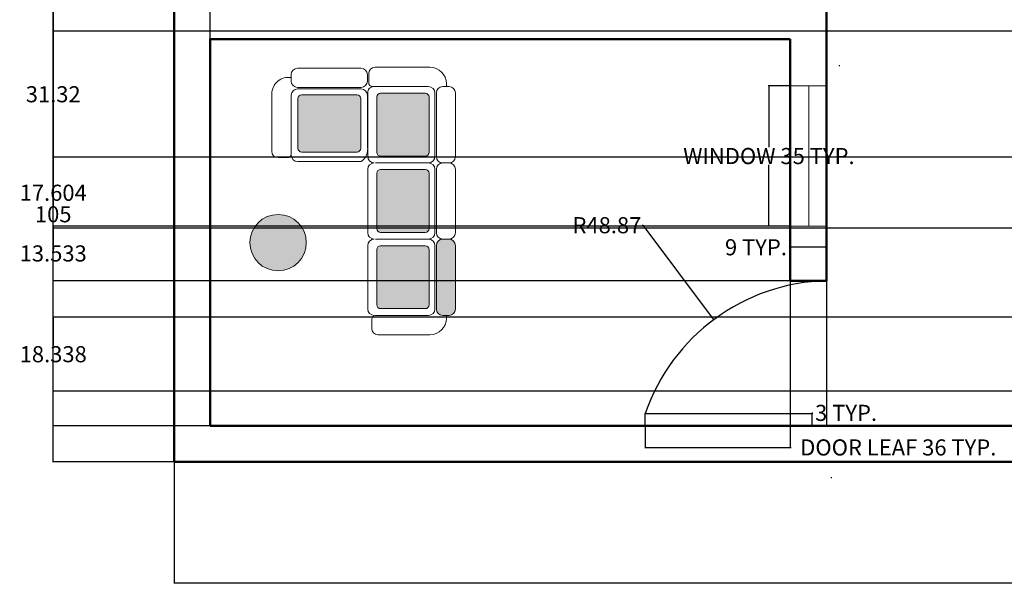
# Model space of a CAD drawing. Units: inches. Extents: x 1454 to 2136, y 626 to 1213.
# Tile 1 of 23: x 1454 to 1699, y 626 to 768. Entities that reach past the tile are written whole.
import ezdxf

# ---------------------------------------------------------------- set-up
doc = ezdxf.new("R2010")
doc.units = ezdxf.units.IN
doc.header["$MEASUREMENT"] = 0
for name, color, linetype, lineweight in [('A-ANNO-DIMS', 2, 'Continuous', 18), ('A-DOOR', 3, 'Continuous', 25), ('A-FURN', 9, 'Continuous', 18), ('A-FURN-PATT', 252, 'Continuous', 13), ('A-GLAZ', 4, 'Continuous', 18), ('A-PLNT-PATT', 116, 'Continuous', 13), ('A-WALL', 7, 'Continuous', 50), ('sofa', 4, 'Continuous', 18)]:
    doc.layers.add(name, color=color, linetype=linetype, lineweight=lineweight)
doc.styles.get("Standard").update_dxf_attribs({"font": 'arial.ttf'})
doc.dimstyles.get("Standard").update_dxf_attribs({"dimtxt": 4, "dimasz": 0.18, "dimexe": 0.18, "dimexo": 0.0625, "dimgap": 0.09, "dimtad": 0, "dimtih": 1, "dimtoh": 1, "dimdec": 0, "dimrnd": 6, "dimzin": 0, "dimdsep": 46, "dimlunit": 3, "dimtxsty": 'Standard', "dimcen": 0.09, "dimadec": 0, "dimazin": 0, "dimtfac": 1, "dimtdec": 0, "dimtofl": 0, "dimtmove": 0, "dimatfit": 3, "dimfxl": 1, "dimtolj": 1, "dimtzin": 0, "dimarcsym": 0})

# ---------------------------------------------------------------- blocks, each defined once
blk = doc.blocks.new('A$C611E44E9')
for p, q in [((0.6611, 1.4447), (0.2101, 1.4447)), ((0.7111, 1.3223), (0.7111, 1.3947)), ((0.0084, 1.2424), (0.0084, 0.7424)), ((0.1084, 1.2927), (0.0584, 1.2927)), ((0.0584, 1.2924), (0.1084, 1.2924)), ((0.1584, 1.2424), (0.1584, 0.7424)), ((0.1705, 1.2422), (0.1705, 0.7424)), ((0.6811, 1.2924), (0.2205, 1.2924)), ((0.6811, 1.2924), (0.2205, 1.2924)), ((0.6811, 1.2922), (0.2205, 1.2922)), ((0.2465, 1.2392), (0.6374, 1.2392)), ((0.7418, 0.7424), (0.7418, 1.2422)), ((0.2165, 0.7749), (0.2165, 1.2092)), ((0.6674, 1.2092), (0.6674, 0.7749)), ((0.6374, 0.7449), (0.2465, 0.7449)), ((0, 0.6327), (0, 0.2017)), ((0.1224, 0.6827), (0.05, 0.6827)), ((0.1084, 0.6927), (0.0584, 0.6927)), ((0.0584, 0.6924), (0.1084, 0.6924)), ((0.1524, 0.6527), (0.1524, 0.2121)), ((0.2024, 0.6896), (0.7021, 0.6896)), ((0.6373, 0.6924), (0.2205, 0.6924)), ((0.6373, 0.6924), (0.2205, 0.6924)), ((0.7521, 0.6289), (0.7521, 0.2121)), ((0.7521, 0.6289), (0.7521, 0.2121)), ((0.8021, 0.6896), (1.3018, 0.6896)), ((1.3521, 0.6289), (1.3521, 0.2121)), ((1.3521, 0.6289), (1.3521, 0.2121)), ((1.4021, 0.6896), (1.9018, 0.6896)), ((1.9518, 0.6289), (1.9518, 0.2121)), ((1.952, 0.6289), (1.952, 0.2121)), ((1.982, 0.6589), (2.0543, 0.6589)), ((0.2048, 0.5892), (0.2048, 0.2381)), ((0.6691, 0.6192), (0.2348, 0.6192)), ((0.6991, 0.2381), (0.6991, 0.5892)), ((0.8045, 0.5892), (0.8045, 0.2381)), ((1.2688, 0.6192), (0.8345, 0.6192)), ((1.2988, 0.2381), (1.2988, 0.5892)), ((1.4045, 0.5892), (1.4045, 0.2381)), ((1.8688, 0.6192), (1.4345, 0.6192)), ((1.8988, 0.2381), (1.8988, 0.5892)), ((2.1043, 0.6089), (2.1043, 0.2017)), ((0.7021, 0.1621), (0.2024, 0.1621)), ((0.2348, 0.2081), (0.6691, 0.2081)), ((1.3018, 0.1621), (0.8021, 0.1621)), ((0.8345, 0.2081), (1.2688, 0.2081)), ((1.9018, 0.1621), (1.4021, 0.1621)), ((1.4345, 0.2081), (1.8688, 0.2081)), ((0.1524, 0.05), (0.1524, 0.1)), ((0.7024, 0.15), (0.2024, 0.15)), ((0.7521, 0.05), (0.7521, 0.1)), ((0.7524, 0.1), (0.7524, 0.05)), ((1.3021, 0.15), (0.8021, 0.15)), ((1.3521, 0.05), (1.3521, 0.1)), ((1.3524, 0.1), (1.3524, 0.05)), ((1.9021, 0.15), (1.4021, 0.15)), ((1.952, 0.05), (1.952, 0.1)), ((1.9521, 0.1), (1.9521, 0.05)), ((0.13, 0.0717), (0.15, 0.0717)), ((0.7024, 0), (0.2024, 0)), ((1.3021, 0), (0.8021, 0)), ((1.9021, 0), (1.4021, 0)), ((1.9743, 0.0717), (1.9543, 0.0717))]:
    blk.add_line(p, q)
for centre, radius, start, end in [((0.2101, 1.3147), 0.13, 90, 189.86144), ((0.6611, 1.3947), 0.05, 0, 90), ((0.6811, 1.3223), 0.03, 270, 0), ((0.0584, 1.2424), 0.05, 90, 180), ((0.1084, 1.2424), 0.05, 0, 90), ((0.2205, 1.2422), 0.05, 90, 180), ((0.2465, 1.2092), 0.03, 90, 180), ((0.6374, 1.2092), 0.03, 0, 90), ((0.6918, 1.2422), 0.05, 0, 90), ((0.2465, 0.7749), 0.03, 180, 270), ((0.6374, 0.7749), 0.03, 270, 0), ((0.0584, 0.7424), 0.05, 180, 270), ((0.1084, 0.7424), 0.05, 270, 0), ((0.2205, 0.7424), 0.05, 180, 270), ((0.653, 0.796), 0.1037, 267.24891, 328.87945), ((0.05, 0.6327), 0.05, 90, 180), ((0.1224, 0.6527), 0.03, 0, 90), ((0.1981, 0.6441), 0.0458, 84.66489, 178.99029), ((0.7021, 0.6396), 0.05, 0, 90), ((0.8021, 0.6396), 0.05, 90, 180), ((1.3018, 0.6396), 0.05, 0, 90), ((1.4021, 0.6396), 0.05, 90, 180), ((1.9018, 0.6396), 0.05, 0, 90), ((1.982, 0.6289), 0.03, 90, 180), ((2.0543, 0.6089), 0.05, 0, 90), ((0.2348, 0.5892), 0.03, 90, 180), ((0.6691, 0.5892), 0.03, 0, 90), ((0.8345, 0.5892), 0.03, 90, 180), ((1.2688, 0.5892), 0.03, 0, 90), ((1.4345, 0.5892), 0.03, 90, 180), ((1.8688, 0.5892), 0.03, 0, 90), ((0.2348, 0.2381), 0.03, 180, 270), ((0.6691, 0.2381), 0.03, 270, 0), ((0.8345, 0.2381), 0.03, 180, 270), ((1.2688, 0.2381), 0.03, 270, 0), ((1.4345, 0.2381), 0.03, 180, 270), ((1.8688, 0.2381), 0.03, 270, 0), ((0.13, 0.2017), 0.13, 180, 270), ((0.2024, 0.2121), 0.05, 180, 270), ((0.7021, 0.2121), 0.05, 270, 0), ((0.8021, 0.2121), 0.05, 180, 270), ((1.3018, 0.2121), 0.05, 270, 0), ((1.4021, 0.2121), 0.05, 180, 270), ((1.9018, 0.2121), 0.05, 270, 0), ((1.9743, 0.2017), 0.13, 270, 0), ((0.2024, 0.1), 0.05, 90, 180), ((0.7024, 0.1), 0.05, 0, 90), ((0.8021, 0.1), 0.05, 90, 180), ((1.3021, 0.1), 0.05, 0, 90), ((1.4021, 0.1), 0.05, 90, 180), ((1.9021, 0.1), 0.05, 0, 90), ((0.2024, 0.05), 0.05, 180, 270), ((0.7024, 0.05), 0.05, 270, 0), ((0.8021, 0.05), 0.05, 180, 270), ((1.3021, 0.05), 0.05, 270, 0), ((1.4021, 0.05), 0.05, 180, 270), ((1.9021, 0.05), 0.05, 270, 0)]:
    blk.add_arc(centre, radius, start, end)
blk = doc.blocks.new('WIN-34_84')
blk.add_line((34.84, 4.31), (0, 4.31))
blk.add_lwpolyline([(34.84, 0), (0, 0), (0, 9), (34.84, 9)], close=True)
blk = doc.blocks.new('DOOR-LEAF-36')
blk.add_lwpolyline([(-36, 3), (0, 3), (0, 0), (-36, 0)], close=True)
blk = doc.blocks.new('*D15')
at = {"layer": 'A-ANNO-DIMS', "color": 0, "lineweight": -2, "transparency": 16777216}
for p, q in [((1609.56, 667.22), (1609.56, 661.7)), ((1645.56, 667.22), (1645.56, 661.7)), ((1609.74, 661.88), (1645.38, 661.88)), ((1645.56, 661.88), (1645.74, 661.88))]:
    blk.add_line(p, q, dxfattribs=at)
at = {"layer": 'A-ANNO-DIMS', "color": 0, "transparency": 16777216}
for points in [[(1609.74, 661.91), (1609.74, 661.85), (1609.56, 661.88)], [(1645.38, 661.91), (1645.38, 661.85), (1645.56, 661.88)]]:
    blk.add_solid(points, dxfattribs=at)
at = {"layer": 'Defpoints', "color": 0, "transparency": 16777216}
for p in [(1609.56, 667.28), (1645.56, 667.28), (1645.56, 661.88)]:
    blk.add_point(p, dxfattribs=at)
at = {"layer": 'A-ANNO-DIMS', "color": 0, "transparency": 16777216, "insert": (1672.38, 661.88), "char_height": 4, "attachment_point": 5}
blk.add_mtext('\\A1;DOOR LEAF 36 TYP.', dxfattribs=at)
blk = doc.blocks.new('*D16')
at = {"layer": 'A-ANNO-DIMS', "color": 0, "lineweight": -2, "transparency": 16777216}
for p, q in [((1645.62, 670.28), (1651.14, 670.28)), ((1650.96, 670.28), (1650.96, 670.46)), ((1650.96, 670.46), (1651.14, 670.46)), ((1650.96, 667.46), (1650.96, 670.1)), ((1645.62, 667.28), (1651.14, 667.28))]:
    blk.add_line(p, q, dxfattribs=at)
at = {"layer": 'A-ANNO-DIMS', "color": 0, "transparency": 16777216}
for points in [[(1650.93, 670.1), (1650.99, 670.1), (1650.96, 670.28)], [(1650.93, 667.46), (1650.99, 667.46), (1650.96, 667.28)]]:
    blk.add_solid(points, dxfattribs=at)
at = {"layer": 'Defpoints', "color": 0, "transparency": 16777216}
for p in [(1645.56, 670.28), (1650.96, 670.28), (1645.56, 667.28)]:
    blk.add_point(p, dxfattribs=at)
at = {"layer": 'A-ANNO-DIMS', "color": 0, "transparency": 16777216, "insert": (1659.41, 670.46), "char_height": 4, "attachment_point": 5}
blk.add_mtext('\\A1;3 TYP.', dxfattribs=at)
blk = doc.blocks.new('*D17')
at = {"layer": 'A-ANNO-DIMS', "color": 0, "lineweight": -2, "transparency": 16777216}
for p, q in [((1645.42, 751.66), (1640.07, 751.66)), ((1640.25, 751.48), (1640.25, 736.4)), ((1640.25, 717), (1640.25, 732.07)), ((1645.42, 716.82), (1640.07, 716.82))]:
    blk.add_line(p, q, dxfattribs=at)
at = {"layer": 'A-ANNO-DIMS', "color": 0, "transparency": 16777216}
for points in [[(1640.22, 751.48), (1640.28, 751.48), (1640.25, 751.66)], [(1640.22, 717), (1640.28, 717), (1640.25, 716.82)]]:
    blk.add_solid(points, dxfattribs=at)
at = {"layer": 'Defpoints', "color": 0, "transparency": 16777216}
for p in [(1640.25, 751.66), (1645.48, 751.66), (1645.48, 716.82)]:
    blk.add_point(p, dxfattribs=at)
at = {"layer": 'A-ANNO-DIMS', "color": 0, "transparency": 16777216, "insert": (1640.25, 734.24), "char_height": 4, "attachment_point": 5}
blk.add_mtext('\\A1;WINDOW 35 TYP.', dxfattribs=at)
blk = doc.blocks.new('*D18')
at = {"layer": 'A-ANNO-DIMS', "color": 0, "lineweight": -2, "transparency": 16777216}
for p, q in [((1645.48, 716.75), (1645.48, 711.41)), ((1654.48, 716.75), (1654.48, 711.41)), ((1645.48, 711.59), (1645.3, 711.59)), ((1654.3, 711.59), (1645.66, 711.59))]:
    blk.add_line(p, q, dxfattribs=at)
at = {"layer": 'A-ANNO-DIMS', "color": 0, "transparency": 16777216}
for points in [[(1645.66, 711.62), (1645.66, 711.56), (1645.48, 711.59)], [(1654.3, 711.62), (1654.3, 711.56), (1654.48, 711.59)]]:
    blk.add_solid(points, dxfattribs=at)
at = {"layer": 'Defpoints', "color": 0, "transparency": 16777216}
for p in [(1645.48, 716.82), (1654.48, 716.82), (1645.48, 711.59)]:
    blk.add_point(p, dxfattribs=at)
at = {"layer": 'A-ANNO-DIMS', "color": 0, "transparency": 16777216, "insert": (1637.03, 711.59), "char_height": 4, "attachment_point": 5}
blk.add_mtext('\\A1;9 TYP.', dxfattribs=at)
blk = doc.blocks.new('*D27')
at = {"layer": 'A-ANNO-DIMS', "color": 0, "lineweight": -2, "transparency": 16777216}
for p, q in [((2092.56, 703.22), (2092.56, 628.1)), ((1492.56, 658.22), (1492.56, 628.1)), ((1492.74, 628.28), (1788.04, 628.28)), ((2092.38, 628.28), (1797.07, 628.28))]:
    blk.add_line(p, q, dxfattribs=at)
at = {"layer": 'A-ANNO-DIMS', "color": 0, "transparency": 16777216}
for points in [[(1492.74, 628.31), (1492.74, 628.25), (1492.56, 628.28)], [(2092.38, 628.31), (2092.38, 628.25), (2092.56, 628.28)]]:
    blk.add_solid(points, dxfattribs=at)
at = {"layer": 'Defpoints', "color": 0, "transparency": 16777216}
for p in [(2092.56, 703.28), (1492.56, 658.28), (2092.56, 628.28)]:
    blk.add_point(p, dxfattribs=at)
at = {"layer": 'A-ANNO-DIMS', "color": 0, "transparency": 16777216, "insert": (1792.56, 628.28), "char_height": 4, "attachment_point": 5}
blk.add_mtext('\\A1;600', dxfattribs=at)
blk = doc.blocks.new('*D28')
at = {"layer": 'A-ANNO-DIMS', "color": 0, "lineweight": -2, "transparency": 16777216}
for p, q in [((1537.49, 1180.28), (1462.37, 1180.28)), ((1462.55, 1180.1), (1462.55, 921.41)), ((1462.55, 658.46), (1462.55, 917.15)), ((1492.49, 658.28), (1462.37, 658.28))]:
    blk.add_line(p, q, dxfattribs=at)
at = {"layer": 'A-ANNO-DIMS', "color": 0, "transparency": 16777216}
for points in [[(1462.52, 1180.1), (1462.58, 1180.1), (1462.55, 1180.28)], [(1462.52, 658.46), (1462.58, 658.46), (1462.55, 658.28)]]:
    blk.add_solid(points, dxfattribs=at)
at = {"layer": 'Defpoints', "color": 0, "transparency": 16777216}
for p in [(1462.55, 1180.28), (1537.56, 1180.28), (1492.56, 658.28)]:
    blk.add_point(p, dxfattribs=at)
at = {"layer": 'A-ANNO-DIMS', "color": 0, "transparency": 16777216, "insert": (1462.55, 919.28), "char_height": 4, "attachment_point": 5}
blk.add_mtext('\\A1;522', dxfattribs=at)
blk = doc.blocks.new('*D41')
at = {"layer": 'A-ANNO-DIMS', "color": 0, "lineweight": -2, "transparency": 16777216}
for p, q in [((1645.49, 772.28), (1462.37, 772.28)), ((1462.55, 772.1), (1462.55, 721.91)), ((1462.55, 667.46), (1462.55, 717.65)), ((1645.49, 667.28), (1462.37, 667.28))]:
    blk.add_line(p, q, dxfattribs=at)
at = {"layer": 'A-ANNO-DIMS', "color": 0, "transparency": 16777216}
for points in [[(1462.52, 772.1), (1462.58, 772.1), (1462.55, 772.28)], [(1462.52, 667.46), (1462.58, 667.46), (1462.55, 667.28)]]:
    blk.add_solid(points, dxfattribs=at)
at = {"layer": 'Defpoints', "color": 0, "transparency": 16777216}
for p in [(1462.55, 772.28), (1645.56, 772.28), (1645.56, 667.28)]:
    blk.add_point(p, dxfattribs=at)
at = {"layer": 'A-ANNO-DIMS', "color": 0, "transparency": 16777216, "insert": (1462.55, 719.78), "char_height": 4, "attachment_point": 5}
blk.add_mtext('\\A1;105', dxfattribs=at)
blk = doc.blocks.new('*D56')
at = {"layer": 'A-ANNO-DIMS', "color": 0, "lineweight": -2, "transparency": 16777216}
for p, q in [((1645.42, 716.82), (1462.37, 716.82)), ((1462.55, 716.64), (1462.55, 712.18)), ((1462.55, 703.46), (1462.55, 707.92)), ((1645.49, 703.28), (1462.37, 703.28))]:
    blk.add_line(p, q, dxfattribs=at)
at = {"layer": 'A-ANNO-DIMS', "color": 0, "transparency": 16777216}
for points in [[(1462.52, 716.64), (1462.58, 716.64), (1462.55, 716.82)], [(1462.52, 703.46), (1462.58, 703.46), (1462.55, 703.28)]]:
    blk.add_solid(points, dxfattribs=at)
at = {"layer": 'Defpoints', "color": 0, "transparency": 16777216}
for p in [(1462.55, 716.82), (1645.48, 716.82), (1645.56, 703.28)]:
    blk.add_point(p, dxfattribs=at)
at = {"layer": 'A-ANNO-DIMS', "color": 0, "transparency": 16777216, "insert": (1462.55, 710.05), "char_height": 4, "attachment_point": 5}
blk.add_mtext('\\A1;13.533', dxfattribs=at)
blk = doc.blocks.new('*D64')
at = {"layer": 'A-ANNO-DIMS', "color": 0, "lineweight": -2, "transparency": 16777216}
for p, q in [((2000.57, 733.92), (1462.37, 733.92)), ((1462.55, 733.74), (1462.55, 727.25)), ((1462.55, 716.5), (1462.55, 722.99)), ((2000.57, 716.32), (1462.37, 716.32))]:
    blk.add_line(p, q, dxfattribs=at)
at = {"layer": 'A-ANNO-DIMS', "color": 0, "transparency": 16777216}
for points in [[(1462.52, 733.74), (1462.58, 733.74), (1462.55, 733.92)], [(1462.52, 716.5), (1462.58, 716.5), (1462.55, 716.32)]]:
    blk.add_solid(points, dxfattribs=at)
at = {"layer": 'Defpoints', "color": 0, "transparency": 16777216}
for p in [(1462.55, 733.92), (2000.63, 733.92), (2000.63, 716.32)]:
    blk.add_point(p, dxfattribs=at)
at = {"layer": 'A-ANNO-DIMS', "color": 0, "transparency": 16777216, "insert": (1462.55, 725.12), "char_height": 4, "attachment_point": 5}
blk.add_mtext('\\A1;17.604', dxfattribs=at)
blk = doc.blocks.new('*D72')
at = {"layer": 'A-ANNO-DIMS', "color": 0, "lineweight": -2, "transparency": 16777216}
for p, q in [((1712.33, 694.2), (1462.37, 694.2)), ((1462.55, 694.02), (1462.55, 687.17)), ((1462.55, 676.04), (1462.55, 682.9)), ((1712.33, 675.86), (1462.37, 675.86))]:
    blk.add_line(p, q, dxfattribs=at)
at = {"layer": 'A-ANNO-DIMS', "color": 0, "transparency": 16777216}
for points in [[(1462.52, 694.02), (1462.58, 694.02), (1462.55, 694.2)], [(1462.52, 676.04), (1462.58, 676.04), (1462.55, 675.86)]]:
    blk.add_solid(points, dxfattribs=at)
at = {"layer": 'Defpoints', "color": 0, "transparency": 16777216}
for p in [(1462.55, 694.2), (1712.39, 694.2), (1712.39, 675.86)]:
    blk.add_point(p, dxfattribs=at)
at = {"layer": 'A-ANNO-DIMS', "color": 0, "transparency": 16777216, "insert": (1462.55, 685.03), "char_height": 4, "attachment_point": 5}
blk.add_mtext('\\A1;18.338', dxfattribs=at)
blk = doc.blocks.new('*D87')
at = {"layer": 'A-ANNO-DIMS', "color": 0, "lineweight": -2, "transparency": 16777216}
for p, q in [((2076.36, 765.24), (1462.37, 765.24)), ((1462.55, 765.06), (1462.55, 751.71)), ((1462.55, 734.1), (1462.55, 747.45)), ((2081.97, 733.92), (1462.37, 733.92))]:
    blk.add_line(p, q, dxfattribs=at)
at = {"layer": 'A-ANNO-DIMS', "color": 0, "transparency": 16777216}
for points in [[(1462.52, 765.06), (1462.58, 765.06), (1462.55, 765.24)], [(1462.52, 734.1), (1462.58, 734.1), (1462.55, 733.92)]]:
    blk.add_solid(points, dxfattribs=at)
at = {"layer": 'Defpoints', "color": 0, "transparency": 16777216}
for p in [(1462.55, 765.24), (2076.42, 765.24), (2082.04, 733.92)]:
    blk.add_point(p, dxfattribs=at)
at = {"layer": 'A-ANNO-DIMS', "color": 0, "transparency": 16777216, "insert": (1462.55, 749.58), "char_height": 4, "attachment_point": 5}
blk.add_mtext('\\A1;31.32', dxfattribs=at)
blk = doc.blocks.new('*D88')
at = {"layer": 'A-ANNO-DIMS', "color": 0, "lineweight": -2, "transparency": 16777216}
for p, q in [((1492.56, 658.34), (1492.56, 1210.46)), ((1492.74, 1210.28), (1495.65, 1210.28)), ((1501.38, 1210.28), (1498.46, 1210.28)), ((1501.56, 667.34), (1501.56, 1210.46))]:
    blk.add_line(p, q, dxfattribs=at)
at = {"layer": 'A-ANNO-DIMS', "color": 0, "transparency": 16777216}
for points in [[(1492.74, 1210.31), (1492.74, 1210.25), (1492.56, 1210.28)], [(1501.38, 1210.31), (1501.38, 1210.25), (1501.56, 1210.28)]]:
    blk.add_solid(points, dxfattribs=at)
at = {"layer": 'Defpoints', "color": 0, "transparency": 16777216}
for p in [(1501.56, 1210.28), (1501.56, 667.28), (1492.56, 658.28)]:
    blk.add_point(p, dxfattribs=at)
at = {"layer": 'A-ANNO-DIMS', "color": 0, "transparency": 16777216, "insert": (1497.06, 1210.28), "char_height": 4, "attachment_point": 5}
blk.add_mtext('\\A1;9', dxfattribs=at)
blk = doc.blocks.new('*D91')
at = {"layer": 'A-ANNO-DIMS', "color": 0, "lineweight": -2, "transparency": 16777216}
for p, q in [((1608.71, 823.38), (1608.89, 823.38)), ((1608.89, 823.38), (1627.11, 798.53)), ((1657.68, 756.72), (1657.86, 756.72)), ((1657.77, 756.63), (1657.77, 756.81))]:
    blk.add_line(p, q, dxfattribs=at)
at = {"layer": 'A-ANNO-DIMS', "color": 0, "transparency": 16777216}
blk.add_solid([(1627.13, 798.54), (1627.09, 798.51), (1627.22, 798.38)], dxfattribs=at)
at = {"layer": 'Defpoints', "color": 0, "transparency": 16777216}
for p in [(1627.22, 798.38), (1657.77, 756.72)]:
    blk.add_point(p, dxfattribs=at)
at = {"layer": 'A-ANNO-DIMS', "color": 0, "transparency": 16777216, "insert": (1599.95, 823.38), "char_height": 4, "attachment_point": 5}
blk.add_mtext('\\A1;R51.66', dxfattribs=at)
blk = doc.blocks.new('*D98')
at = {"layer": 'A-ANNO-DIMS', "color": 0, "lineweight": -2, "transparency": 16777216}
for p, q in [((1608.79, 717.06), (1608.97, 717.06)), ((1608.97, 717.06), (1626.42, 693.71)), ((1655.7, 654.42), (1655.88, 654.42)), ((1655.79, 654.33), (1655.79, 654.51))]:
    blk.add_line(p, q, dxfattribs=at)
at = {"layer": 'A-ANNO-DIMS', "color": 0, "transparency": 16777216}
blk.add_solid([(1626.44, 693.73), (1626.39, 693.7), (1626.52, 693.57)], dxfattribs=at)
at = {"layer": 'Defpoints', "color": 0, "transparency": 16777216}
for p in [(1626.52, 693.57), (1655.79, 654.42)]:
    blk.add_point(p, dxfattribs=at)
at = {"layer": 'A-ANNO-DIMS', "color": 0, "transparency": 16777216, "insert": (1600.03, 717.06), "char_height": 4, "attachment_point": 5}
blk.add_mtext('\\A1;R48.87', dxfattribs=at)

msp = doc.modelspace()

# ---------------------------------------------------------------- hatches: boundary and pattern name
at = {"layer": 'A-FURN-PATT'}
h = msp.add_hatch(dxfattribs=at)
h.set_pattern_fill('ESCHER', color=256)
h.paths.add_polyline_path([(1511.3761, 923.7174, 1), (1525.379, 923.7174, 1)])
h.paths.add_polyline_path([(1525.379, 816.0542, 1), (1511.3761, 816.0542, 1)])
h.paths.add_polyline_path([(1525.379, 712.7345, 1), (1511.3761, 712.7345, 1)])
h.paths.add_polyline_path([(2070.5057, 794.3402, 1), (2056.5027, 794.3402, 1)])
h.paths.add_polyline_path([(2005.868, 1014.5578, 1), (1991.8651, 1014.5578, 1)])
h.paths.add_polyline_path([(1994.0647, 1066.7584, 1), (2008.0677, 1066.7584, 1)])
h.paths.add_polyline_path([(1919.5492, 1065.3848, 1), (1933.5521, 1065.3848, 1)])
h.paths.add_polyline_path([(1936.8517, 1013.7336, 1), (1922.8488, 1013.7336, 1)])
h.paths.add_polyline_path([(1824.6062, 1109.1557, 1), (1838.6091, 1109.1557, 1)])
h = msp.add_hatch(color=256, dxfattribs=at)
h.dxf.hatch_style = 1
h.paths.add_polyline_path([(1855.0231, 1089.5248, 0.41421356), (1850.0231, 1094.5248), (1811.2288, 1094.5248, 0.41421356), (1806.2288, 1089.5248), (1806.2288, 1083.6305, 0.41421356), (1811.2288, 1078.6305), (1850.0231, 1078.6305, 0.41421356), (1855.0231, 1083.6305)])
h.paths.add_polyline_path([(1939.0638, 1089.4209), (1938.9354, 1078.7354, -0.20858653), (1943.5258, 1076.1857), (1952.7682, 1081.5837, 0.24238954)])
h.paths.add_polyline_path([(1939.0638, 1089.4209, 0.00796483), (1938.5148, 1089.4363), (1928.0643, 1089.5619), (1927.936, 1078.8906), (1938.3866, 1078.765, -0.02092855), (1938.9354, 1078.7354)])
h.paths.add_polyline_path([(1928.0643, 1089.5619), (1916.0797, 1089.706), (1916.0698, 1088.8851), (1917.241, 1088.8711, -0.41420041), (1917.7276, 1088.3726), (1917.6308, 1080.3281, -0.41422672), (1917.1324, 1079.8415), (1915.9612, 1079.8556), (1915.9573, 1079.5272, 0.41420799), (1916.4439, 1079.0288), (1927.936, 1078.8906)])
h.paths.add_polyline_path([(1917.7276, 1088.3726, 0.41420041), (1917.241, 1088.8711), (1914.9926, 1088.8981, 0.41421356), (1914.4941, 1088.4115), (1914.3974, 1080.367, 0.41421356), (1914.884, 1079.8686), (1917.1324, 1079.8415, 0.41422672), (1917.6308, 1080.3281)])
h.paths.add_polyline_path([(1928.0939, 1092.0245), (1916.6018, 1092.1627, 0.41422672), (1916.1033, 1091.6761), (1916.0797, 1089.706), (1928.0643, 1089.5619)])
h.paths.add_polyline_path([(1939.0935, 1091.8846, 0.00696804), (1938.5445, 1091.8989), (1928.0939, 1092.0245), (1928.0643, 1089.5619), (1938.5148, 1089.4363, -0.00796483), (1939.0638, 1089.4209)])
h.paths.add_polyline_path([(1939.0935, 1091.8846), (1939.0638, 1089.4209, -0.24238954), (1952.7682, 1081.5837), (1954.897, 1082.827, 0.24500473)])
h.paths.add_polyline_path([(1952.7682, 1081.5837), (1943.5258, 1076.1857, -0.16768112), (1944.8746, 1072.1191), (1944.8073, 1066.5201), (1955.4785, 1066.3918), (1955.5459, 1071.9909, 0.14799784)])
h.paths.add_polyline_path([(1954.897, 1082.827), (1952.7682, 1081.5837, -0.14799784), (1955.5459, 1071.9909), (1955.4785, 1066.3918), (1957.9412, 1066.3622), (1958.0085, 1071.9612, 0.14649407)])
h.paths.add_polyline_path([(1955.4785, 1066.3918), (1944.8073, 1066.5201), (1944.675, 1055.5205, 0.41421356), (1945.1616, 1055.0221), (1945.49, 1055.0181), (1945.5041, 1056.1893, -0.41421356), (1946.0025, 1056.6759), (1954.047, 1056.5792, -0.41421356), (1954.5336, 1056.0807), (1954.5195, 1054.9096), (1955.3404, 1054.8997)])
h.paths.add_polyline_path([(1954.5336, 1056.0807, 0.41421356), (1954.047, 1056.5792), (1946.0025, 1056.6759, 0.41421356), (1945.5041, 1056.1893), (1945.49, 1055.0181), (1945.477, 1053.9409, 0.41422115), (1945.9636, 1053.4425), (1954.0081, 1053.3458, 0.41420598), (1954.5066, 1053.8324)])
h.paths.add_polyline_path([(1957.9412, 1066.3622), (1955.4785, 1066.3918), (1955.3404, 1054.8997), (1957.3105, 1054.876, 0.41421356), (1957.8089, 1055.3626)])
h.paths.add_polyline_path([(1974.6911, 1066.3918), (1972.2285, 1066.3622), (1972.3608, 1055.3626, 0.41421356), (1972.8592, 1054.876), (1974.8293, 1054.8997)])
h.paths.add_polyline_path([(1985.3624, 1066.5201), (1974.6911, 1066.3918), (1974.8293, 1054.8997), (1975.6501, 1054.9096), (1975.6361, 1056.0807, -0.41421356), (1976.1227, 1056.5792), (1984.1672, 1056.6759, -0.41421356), (1984.6656, 1056.1893), (1984.6797, 1055.0181), (1985.008, 1055.0221, 0.41421356), (1985.4946, 1055.5205)])
h.paths.add_polyline_path([(1984.6656, 1056.1893, 0.41421356), (1984.1672, 1056.6759), (1976.1227, 1056.5792, 0.41421356), (1975.6361, 1056.0807), (1975.6631, 1053.8324, 0.41422115), (1976.1615, 1053.3458), (1984.206, 1053.4425, 0.41420597), (1984.6926, 1053.9409)])
h.paths.add_polyline_path([(1985.2951, 1072.1191, -0.16768112), (1986.6438, 1076.1857), (1977.4014, 1081.5837, 0.14799988), (1974.6238, 1071.9907), (1974.6911, 1066.3918), (1985.3624, 1066.5201)])
h.paths.add_polyline_path([(1977.4014, 1081.5837), (1975.2727, 1082.827, 0.14649407), (1972.1612, 1071.9612), (1972.2285, 1066.3622), (1974.6911, 1066.3918), (1974.6238, 1071.9907, -0.14799988)])
h.paths.add_polyline_path([(1991.1058, 1089.4209, 0.24238954), (1977.4014, 1081.5837), (1986.6438, 1076.1857, -0.20858653), (1991.2343, 1078.7354)])
h.paths.add_polyline_path([(1991.1058, 1089.4209), (1991.0762, 1091.8846, 0.24500473), (1975.2727, 1082.827), (1977.4014, 1081.5837, -0.24238954)])
h.paths.add_polyline_path([(2002.1053, 1089.5619), (1991.6547, 1089.4363, 0.00796283), (1991.1058, 1089.4209), (1991.2343, 1078.7354, -0.02092855), (1991.783, 1078.765), (2002.2336, 1078.8906)])
h.paths.add_polyline_path([(2002.0757, 1092.0245), (1991.6251, 1091.8989, 0.00696804), (1991.0762, 1091.8846), (1991.1058, 1089.4209, -0.00796283), (1991.6547, 1089.4363), (2002.1053, 1089.5619)])
h.paths.add_polyline_path([(2014.0663, 1091.6761, 0.4142004), (2013.5679, 1092.1627), (2002.0757, 1092.0245), (2002.1053, 1089.5619), (2014.09, 1089.706)])
h.paths.add_polyline_path([(2012.4421, 1088.3726, -0.41422672), (2012.9287, 1088.8711), (2014.0999, 1088.8851), (2014.09, 1089.706), (2002.1053, 1089.5619), (2002.2336, 1078.8906), (2013.7258, 1079.0288, 0.41421913), (2014.2124, 1079.5273), (2014.2084, 1079.8556), (2013.0373, 1079.8415, -0.4142004), (2012.5388, 1080.3281)])
h.paths.add_polyline_path([(1986.6438, 1024.0964), (1977.4014, 1029.4944, 0.14799988), (1974.6238, 1019.9014), (1974.6911, 1014.3025), (1985.3624, 1014.4308), (1985.2951, 1020.0298, -0.16768112)])
h.paths.add_polyline_path([(1991.1058, 1037.3316, 0.24238954), (1977.4014, 1029.4944), (1986.6438, 1024.0964, -0.20858653), (1991.2343, 1026.6461)])
h.paths.add_polyline_path([(2002.1053, 1037.4726), (1991.6547, 1037.347, 0.00796283), (1991.1058, 1037.3316), (1991.2343, 1026.6461, -0.02092855), (1991.783, 1026.6757), (2002.2336, 1026.8013)])
h.paths.add_polyline_path([(2012.4421, 1036.2833, -0.41422672), (2012.9287, 1036.7818), (2014.0999, 1036.7958), (2014.09, 1037.6167), (2002.1053, 1037.4726), (2002.2336, 1026.8013), (2013.7258, 1026.9395, 0.41421913), (2014.2124, 1027.438), (2014.2084, 1027.7663), (2013.0373, 1027.7522, -0.4142004), (2012.5388, 1028.2388)])
h.paths.add_polyline_path([(2015.6755, 1036.3222, 0.41421356), (2015.1771, 1036.8088), (2012.9287, 1036.7818, 0.41422672), (2012.4421, 1036.2833), (2012.5388, 1028.2388, 0.4142004), (2013.0373, 1027.7522), (2015.2856, 1027.7793, 0.41421356), (2015.7722, 1028.2777)])
h.paths.add_polyline_path([(1985.3624, 1014.4308), (1974.6911, 1014.3025), (1974.8293, 1002.8104), (1975.6501, 1002.8203), (1975.6361, 1003.9914, -0.41421356), (1976.1227, 1004.4899), (1984.1672, 1004.5866, -0.41421356), (1984.6656, 1004.1), (1984.6797, 1002.9288), (1985.008, 1002.9328, 0.41421356), (1985.4946, 1003.4312)])
h.paths.add_polyline_path([(1984.6656, 1004.1, 0.41421356), (1984.1672, 1004.5866), (1976.1227, 1004.4899, 0.41421356), (1975.6361, 1003.9914), (1975.6631, 1001.743, 0.41422115), (1976.1615, 1001.2564), (1984.206, 1001.3532, 0.41420598), (1984.6926, 1001.8516)])
h.paths.add_polyline_path([(1974.6911, 1014.3025), (1972.2285, 1014.2729), (1972.3608, 1003.2733, 0.41421356), (1972.8592, 1002.7867), (1974.8293, 1002.8104)])
h.paths.add_polyline_path([(1974.6238, 1019.9014, -0.14799988), (1977.4014, 1029.4944), (1975.2727, 1030.7376, 0.14649407), (1972.1612, 1019.8719), (1972.2285, 1014.2729), (1974.6911, 1014.3025)])
h.paths.add_polyline_path([(1991.1058, 1037.3316), (1991.0762, 1039.7953, 0.24500473), (1975.2727, 1030.7376), (1977.4014, 1029.4944, -0.24238954)])
h.paths.add_polyline_path([(2002.0757, 1039.9352), (1991.6251, 1039.8096, 0.00696804), (1991.0762, 1039.7953), (1991.1058, 1037.3316, -0.00796283), (1991.6547, 1037.347), (2002.1053, 1037.4726)])
h.paths.add_polyline_path([(2014.0663, 1039.5868, 0.4142004), (2013.5679, 1040.0734), (2002.0757, 1039.9352), (2002.1053, 1037.4726), (2014.09, 1037.6167)])
h.paths.add_polyline_path([(1955.5459, 1019.9016, 0.14799784), (1952.7682, 1029.4944), (1943.5258, 1024.0964, -0.16768112), (1944.8746, 1020.0298), (1944.8073, 1014.4308), (1955.4785, 1014.3025)])
h.paths.add_polyline_path([(1955.4785, 1014.3025), (1944.8073, 1014.4308), (1944.675, 1003.4312, 0.41421356), (1945.1616, 1002.9328), (1945.49, 1002.9288), (1945.5041, 1004.1, -0.41421356), (1946.0025, 1004.5866), (1954.047, 1004.4899, -0.41421356), (1954.5336, 1003.9914), (1954.5195, 1002.8203), (1955.3404, 1002.8104)])
h.paths.add_polyline_path([(1939.0638, 1037.3316), (1938.9354, 1026.6461, -0.20858653), (1943.5258, 1024.0964), (1952.7682, 1029.4944, 0.24238954)])
h.paths.add_polyline_path([(1939.0638, 1037.3316, 0.00796483), (1938.5148, 1037.347), (1928.0643, 1037.4726), (1927.936, 1026.8013), (1938.3866, 1026.6757, -0.02092855), (1938.9354, 1026.6461)])
h.paths.add_polyline_path([(1928.0643, 1037.4726), (1916.0797, 1037.6167), (1916.0698, 1036.7958), (1917.241, 1036.7818, -0.41420041), (1917.7276, 1036.2833), (1917.6308, 1028.2388, -0.41422672), (1917.1324, 1027.7522), (1915.9612, 1027.7663), (1915.9573, 1027.4379, 0.41420799), (1916.4439, 1026.9395), (1927.936, 1026.8013)])
h.paths.add_polyline_path([(1917.7276, 1036.2833, 0.41420041), (1917.241, 1036.7818), (1914.9926, 1036.8088, 0.41421356), (1914.4941, 1036.3222), (1914.3974, 1028.2777, 0.41421356), (1914.884, 1027.7793), (1917.1324, 1027.7522, 0.41422672), (1917.6308, 1028.2388)])
h.paths.add_polyline_path([(1928.0939, 1039.9352), (1916.6018, 1040.0734, 0.41422672), (1916.1033, 1039.5868), (1916.0797, 1037.6167), (1928.0643, 1037.4726)])
h.paths.add_polyline_path([(1939.0935, 1039.7953, 0.00696804), (1938.5445, 1039.8096), (1928.0939, 1039.9352), (1928.0643, 1037.4726), (1938.5148, 1037.347, -0.00796483), (1939.0638, 1037.3316)])
h.paths.add_polyline_path([(1939.0935, 1039.7953), (1939.0638, 1037.3316, -0.24238954), (1952.7682, 1029.4944), (1954.897, 1030.7376, 0.24500473)])
h.paths.add_polyline_path([(1954.897, 1030.7376), (1952.7682, 1029.4944, -0.14799784), (1955.5459, 1019.9016), (1955.4785, 1014.3025), (1957.9412, 1014.2729), (1958.0085, 1019.8719, 0.14649407)])
h.paths.add_polyline_path([(1957.9412, 1014.2729), (1955.4785, 1014.3025), (1955.3404, 1002.8104), (1957.3105, 1002.7867, 0.41421356), (1957.8089, 1003.2733)])
h.paths.add_polyline_path([(1954.5336, 1003.9914, 0.41421356), (1954.047, 1004.4899), (1946.0025, 1004.5866, 0.41421356), (1945.5041, 1004.1), (1945.49, 1002.9288), (1945.477, 1001.8516, 0.41422115), (1945.9636, 1001.3532), (1954.0081, 1001.2564, 0.41420598), (1954.5066, 1001.743)])
h.paths.add_polyline_path([(1997.553, 886.9384), (1981.0334, 886.9384), (1981.0334, 876.3409, 0.41421356), (1984.1503, 873.224), (1996.6179, 873.224, 0.41421356), (1999.7348, 876.3409), (1998.488, 876.3409, -0.41421356), (1997.553, 877.276)])
h.paths.add_polyline_path([(1981.0334, 886.9384), (1964.5139, 886.9384), (1964.5139, 877.276, -0.41421356), (1963.5788, 876.3409), (1962.3321, 876.3409, 0.41421356), (1965.449, 873.224), (1977.9165, 873.224, 0.41421356), (1981.0334, 876.3409)])
h.paths.add_polyline_path([(1964.5139, 886.9384), (1964.5139, 887.25, 0.47353022), (1963.4209, 888.1978, -0.46345458), (1962.3321, 889.1202), (1962.3321, 890.6786), (1962.3321, 892.5488), (1961.0853, 892.5488, 0.41421356), (1960.1503, 891.6137), (1960.1503, 877.276, 0.41421356), (1961.0853, 876.3409), (1963.5788, 876.3409, 0.41421356), (1964.5139, 877.276)])
h.paths.add_polyline_path([(1999.7348, 892.5488), (1999.7348, 893.7955, 0.41421356), (1998.7997, 894.7306), (1963.2672, 894.7306, 0.41421356), (1962.3321, 893.7955), (1962.3321, 892.5488), (1962.3321, 890.3669, 0.41421356), (1963.2672, 889.4319), (1998.7997, 889.4319, 0.41421356), (1999.7348, 890.3669), (1999.7348, 890.6786)])
h.paths.add_polyline_path([(2001.9166, 891.6137, 0.41421356), (2000.9815, 892.5488), (1999.7348, 892.5488), (1999.7348, 890.6786), (1999.7348, 890.3669), (1999.7348, 889.1202, -0.41421356), (1998.7997, 888.1851), (1998.488, 888.1851, 0.41421356), (1997.553, 887.25), (1997.553, 877.276, 0.41421356), (1998.488, 876.3409), (1999.7348, 876.3409), (2000.9815, 876.3409, 0.41421356), (2001.9166, 877.276)])
h.paths.add_polyline_path([(1999.7348, 889.1202), (1999.7348, 890.3669, -0.41421356), (1998.7997, 889.4319), (1963.2672, 889.4319, -0.41421356), (1962.3321, 890.3669), (1962.3321, 889.1202, 0.46345458), (1963.4209, 888.1978, -0.45647258), (1964.5139, 887.3025), (1964.5139, 886.9384), (1997.553, 886.9384), (1997.553, 887.25, -0.41421356), (1998.488, 888.1851), (1998.7997, 888.1851, 0.41421356)])
h.paths.add_polyline_path([(1540.5701, 966.1379, 0.41421356), (1538.9915, 967.7165), (1523.2061, 967.7165, 0.41421356), (1521.6275, 966.1379), (1521.6275, 964.5679, 0.41579661), (1523.2061, 962.9808), (1538.9915, 962.9808, 0.41421356), (1540.5701, 964.5594)])
h.paths.add_polyline_path([(1538.9151, 960.1995, 0.41421356), (1537.968, 961.1466), (1524.2565, 961.1466, 0.41421356), (1523.3094, 960.1995), (1523.3094, 947.859, 0.41421356), (1524.2565, 946.9119), (1537.968, 946.9119, 0.41421356), (1538.9151, 947.859)])
h.paths.add_polyline_path([(1555.8609, 960.5704, 0.41421356), (1554.9138, 961.5176), (1543.8299, 961.5176, 0.41421356), (1542.8828, 960.5704), (1542.8828, 946.859, 0.41421356), (1543.8299, 945.9119), (1554.9138, 945.9119, 0.41421356), (1555.8609, 946.859)])
h.paths.add_polyline_path([(1555.8609, 941.6364, 0.41421356), (1554.9138, 942.5835), (1543.8299, 942.5835, 0.41421356), (1542.8828, 941.6364), (1542.8828, 927.9249, 0.41421356), (1543.8299, 926.9778), (1554.9138, 926.9778, 0.41421356), (1555.8609, 927.9249)])
h.paths.add_polyline_path([(1555.8609, 922.6938, 0.41421356), (1554.9138, 923.6409), (1543.8299, 923.6409, 0.41421356), (1542.8828, 922.6938), (1542.8828, 908.9824, 0.41421356), (1543.8299, 908.0352), (1554.9138, 908.0352, 0.41421356), (1555.8609, 908.9824)])
h.paths.add_polyline_path([(1555.8609, 815.2921, 0.41421356), (1554.9138, 816.2392), (1543.8299, 816.2392, 0.41421356), (1542.8828, 815.2921), (1542.8828, 801.5806, 0.41421356), (1543.8299, 800.6335), (1554.9138, 800.6335, 0.41421356), (1555.8609, 801.5806)])
h.paths.add_polyline_path([(1555.8609, 834.2346, 0.41421356), (1554.9138, 835.1818), (1543.8299, 835.1818, 0.41421356), (1542.8828, 834.2346), (1542.8828, 820.5232, 0.41421356), (1543.8299, 819.576), (1554.9138, 819.576, 0.41421356), (1555.8609, 820.5232)])
h.paths.add_polyline_path([(1555.8609, 853.1687, 0.41421356), (1554.9138, 854.1158), (1543.8299, 854.1158, 0.41421356), (1542.8828, 853.1687), (1542.8828, 839.4572, 0.41421356), (1543.8299, 838.5101), (1554.9138, 838.5101, 0.41421356), (1555.8609, 839.4572)])
h.paths.add_polyline_path([(1538.9151, 852.7977, 0.41421356), (1537.968, 853.7448), (1524.2565, 853.7448, 0.41421356), (1523.3094, 852.7977), (1523.3094, 840.4573, 0.41421356), (1524.2565, 839.5101), (1537.968, 839.5101, 0.41421356), (1538.9151, 840.4573)])
h.paths.add_polyline_path([(1538.9151, 748.5053, 0.41421356), (1537.968, 749.4524), (1524.2565, 749.4524, 0.41421356), (1523.3094, 748.5053), (1523.3094, 736.1648, 0.41421356), (1524.2565, 735.2177), (1537.968, 735.2177, 0.41421356), (1538.9151, 736.1648)])
h.paths.add_polyline_path([(1555.8609, 748.8763, 0.41421356), (1554.9138, 749.8234), (1543.8299, 749.8234, 0.41421356), (1542.8828, 748.8763), (1542.8828, 735.1648, 0.41421356), (1543.8299, 734.2177), (1554.9138, 734.2177, 0.41421356), (1555.8609, 735.1648)])
h.paths.add_polyline_path([(1555.8609, 729.9422, 0.41421356), (1554.9138, 730.8893), (1543.8299, 730.8893, 0.41421356), (1542.8828, 729.9422), (1542.8828, 716.2308, 0.41421356), (1543.8299, 715.2836), (1554.9138, 715.2836, 0.41421356), (1555.8609, 716.2308)])
h.paths.add_polyline_path([(1555.8609, 710.9996, 0.41421356), (1554.9138, 711.9468), (1543.8299, 711.9468, 0.41421356), (1542.8828, 710.9996), (1542.8828, 697.2882, 0.41421356), (1543.8299, 696.3411), (1554.9138, 696.3411, 0.41421356), (1555.8609, 697.2882)])
h.paths.add_polyline_path([(1562.4308, 712.0232, 0.44500955), (1560.6884, 713.5932), (1559.1098, 713.5932, 0.3840739), (1557.6951, 712.0232), (1557.6951, 696.2377, 0.43158582), (1559.3667, 694.6619), (1560.9452, 694.6619, 0.39705211), (1562.4308, 696.2377)])
h.paths.add_polyline_path([(1559.2737, 713.6017, -0.41421356), (1557.6951, 715.1803), (1557.6951, 730.9658, -0.39284205), (1559.1577, 732.5401, -0.39284205), (1557.6951, 734.1143), (1557.6951, 749.8998, -0.41421356), (1559.2737, 751.4784), (1560.8522, 751.4784, -0.41421356), (1562.4308, 749.8998), (1562.4308, 734.1143, -0.39284205), (1560.9682, 732.5401, -0.39284205), (1562.4308, 730.9658), (1562.4308, 715.1803, -0.41421356), (1560.8522, 713.6017), (1559.2737, 713.5932), (1559.4375, 713.5932, 0.05204098), (1559.1098, 713.5932)])
h.paths.add_polyline_path([(1559.2737, 732.5443), (1559.2737, 732.5358), (1560.8522, 732.5358), (1560.8522, 732.5443)], flags=16)
h.paths.add_polyline_path([(1562.4308, 749.8998, 0.41421356), (1560.8522, 751.4784), (1559.2737, 751.4784, 0.41421356), (1557.6951, 749.8998), (1557.6951, 734.1143, 0.41421356), (1559.2737, 732.5358), (1559.2737, 732.5443, 0.41421356), (1557.6951, 730.9658), (1557.6951, 715.1803, 0.41421356), (1559.2737, 713.6017), (1560.8437, 713.6018, 0.41579661), (1562.4308, 715.1803), (1562.4308, 730.9658, 0.41421356), (1560.8522, 732.5443), (1560.8522, 732.5358, 0.41421356), (1562.4308, 734.1143)])
at = {"layer": 'A-PLNT-PATT'}
h = msp.add_hatch(dxfattribs=at)
h.set_pattern_fill('ESCHER', color=256)
h.paths.add_polyline_path([(1767.2815, 694.0009, 1), (1753.2786, 694.0009, 1)])
h.paths.add_polyline_path([(1578.6873, 1043.8029, 1), (1564.6844, 1043.8029, 1)])

# ---------------------------------------------------------------- linework, layer by layer
at = {"layer": 'A-DOOR'}
for p, q in [((1645.5563, 703.2825), (1645.5563, 667.2825)), ((1654.5563, 703.2825), (1654.5563, 667.2825))]:
    msp.add_line(p, q, dxfattribs=at)
msp.add_arc((1655.7854, 654.4247), 48.8732, 91.440994, 161.066682, dxfattribs=at)
at = {"layer": 'A-FURN'}
msp.add_circle((1518.3775, 712.7345), 7.0015, dxfattribs=at)
at = {"layer": 'A-WALL'}
for p, q in [((1492.5563, 982.2825), (1492.5563, 700.2825)), ((1654.5563, 772.2825), (1654.5563, 703.2825)), ((1645.5563, 763.2825), (1501.5563, 763.2825)), ((1501.5563, 763.2825), (1501.5563, 667.2825)), ((1645.5563, 763.2825), (1645.5563, 703.2825)), ((1501.5563, 703.2825), (1501.5563, 667.2825)), ((1654.5563, 703.2825), (1645.5563, 703.2825)), ((1492.5563, 700.2825), (1492.5563, 658.2825)), ((1774.5563, 667.2825), (1501.5563, 667.2825)), ((1501.5563, 658.2825), (1492.5563, 658.2825)), ((1783.5563, 658.2825), (1501.5563, 658.2825))]:
    msp.add_line(p, q, dxfattribs=at)

# ---------------------------------------------------------------- block references
at = {"layer": 'A-DOOR'}
msp.add_blockref('DOOR-LEAF-36', (1645.5563, 667.2825), dxfattribs=at)
at = {"layer": 'A-GLAZ', "rotation": 89.99999999999984}
msp.add_blockref('WIN-34_84', (1654.4779, 716.8154), dxfattribs=at)
at = {"layer": 'sofa', "xscale": -31.57095925523166, "yscale": 31.57095925523166, "zscale": 31.57095925523166, "rotation": 90}
msp.add_blockref('A$C611E44E9', (1562.4308, 756.2883), dxfattribs=at)

# ---------------------------------------------------------------- dimensions: what is measured, and where the dimension line sits
at = {"layer": 'A-ANNO-DIMS'}
for base, p2, picture, middle in [((1501.5563, 1210.2845), (1501.5563, 667.2825), '*D88', (1497.0563, 1210.2845)), ((2092.5563, 628.2805), (2092.5563, 703.2825), '*D27', (1792.5563, 628.2805))]:
    dim = msp.add_linear_dim(base=base, p1=(1492.5563, 658.2825), p2=p2, dimstyle='Standard', override={"dimdec": 0, "dimlfac": 1, "dimrnd": 0, "dimzin": 0, "dimdsep": 46, "dimlunit": 2}, dxfattribs=at)
    dim.commit()
    dim.dimension.update_dxf_attribs({"geometry": picture, "text_midpoint": middle})
for base, p1, p2, override, picture, middle in [((1462.5543, 1180.2825), (1492.5563, 658.2825), (1537.5563, 1180.2825), {"dimdec": 0, "dimlfac": 1, "dimrnd": 0, "dimzin": 0, "dimdsep": 46, "dimlunit": 2}, '*D28', (1462.5543, 919.2825)), ((1462.5543, 772.2825), (1645.5563, 667.2825), (1645.5563, 772.2825), {"dimdec": 0, "dimlfac": 1, "dimrnd": 0, "dimzin": 0, "dimdsep": 46, "dimlunit": 2}, '*D41', (1462.5543, 719.7825)), ((1462.5543, 765.2409), (2082.0362, 733.9205), (2076.4223, 765.2409), {"dimdec": 2, "dimlfac": 1, "dimrnd": 0, "dimzin": 0, "dimdsep": 46, "dimlunit": 2}, '*D87', (1462.5543, 749.5807)), ((1462.5543, 733.9205), (2000.6276, 716.3161), (2000.6276, 733.9205), {"dimdec": 3, "dimlfac": 1, "dimrnd": 0, "dimzin": 0, "dimdsep": 46, "dimlunit": 2}, '*D64', (1462.5543, 725.1183)), ((1462.5543, 716.8154), (1645.5563, 703.2825), (1645.4779, 716.8154), {"dimdec": 3, "dimlfac": 1, "dimrnd": 0, "dimzin": 0, "dimdsep": 46, "dimlunit": 2}, '*D56', (1462.5543, 710.0489)), ((1462.5543, 694.2005), (1712.3887, 675.8628), (1712.3887, 694.2005), {"dimdec": 3, "dimlfac": 1, "dimrnd": 0, "dimzin": 0, "dimdsep": 46, "dimlunit": 2}, '*D72', (1462.5543, 685.0317))]:
    dim = msp.add_linear_dim(base=base, p1=p1, p2=p2, angle=90, dimstyle='Standard', override=override, dxfattribs=at)
    dim.commit()
    dim.dimension.update_dxf_attribs({"geometry": picture, "text_midpoint": middle})
for center, mpoint, picture, middle in [((1657.7683, 756.7207), (1627.2172, 798.3808), '*D91', (1599.9548, 823.3768)), ((1655.7854, 654.4247), (1626.5229, 693.5693), '*D98', (1600.0324, 717.0561))]:
    dim = msp.add_radius_dim(center=center, mpoint=mpoint, dimstyle='Standard', override={"dimdec": 2, "dimlfac": 1, "dimrnd": 0, "dimzin": 0, "dimdsep": 46, "dimlunit": 2}, dxfattribs=at)
    dim.commit()
    dim.dimension.update_dxf_attribs({"geometry": picture, "text_midpoint": middle, "dimtype": 164})
for base, p1, p2, angle, text, picture, middle in [((1640.2519, 751.6556), (1645.4779, 716.8154), (1645.4779, 751.6556), 90, 'WINDOW <> TYP.', '*D17', (1640.2519, 734.2355)), ((1645.4779, 711.5893), (1654.4779, 716.8154), (1645.4779, 716.8154), 180, '<> TYP.', '*D18', (1637.0265, 711.5893)), ((1650.9563, 670.2825), (1645.5563, 667.2825), (1645.5563, 670.2825), 90, '<> TYP.', '*D16', (1659.4064, 670.4625))]:
    dim = msp.add_linear_dim(base=base, p1=p1, p2=p2, angle=angle, text=text, dimstyle='Standard', override={"dimdec": 0, "dimlfac": 1, "dimrnd": 0, "dimzin": 0, "dimdsep": 46, "dimlunit": 2}, dxfattribs=at)
    dim.commit()
    dim.dimension.update_dxf_attribs({"geometry": picture, "text_midpoint": middle})
dim = msp.add_linear_dim(base=(1645.5563, 661.8825), p1=(1609.5563, 667.2825), p2=(1645.5563, 667.2825), text='DOOR LEAF <> TYP.', dimstyle='Standard', override={"dimdec": 0, "dimlfac": 1, "dimrnd": 0, "dimzin": 0, "dimdsep": 46, "dimlunit": 2}, dxfattribs=at)
dim.commit()
dim.dimension.update_dxf_attribs({"geometry": '*D15', "text_midpoint": (1672.3843, 661.8825)})

doc.saveas('drawing.dxf')
